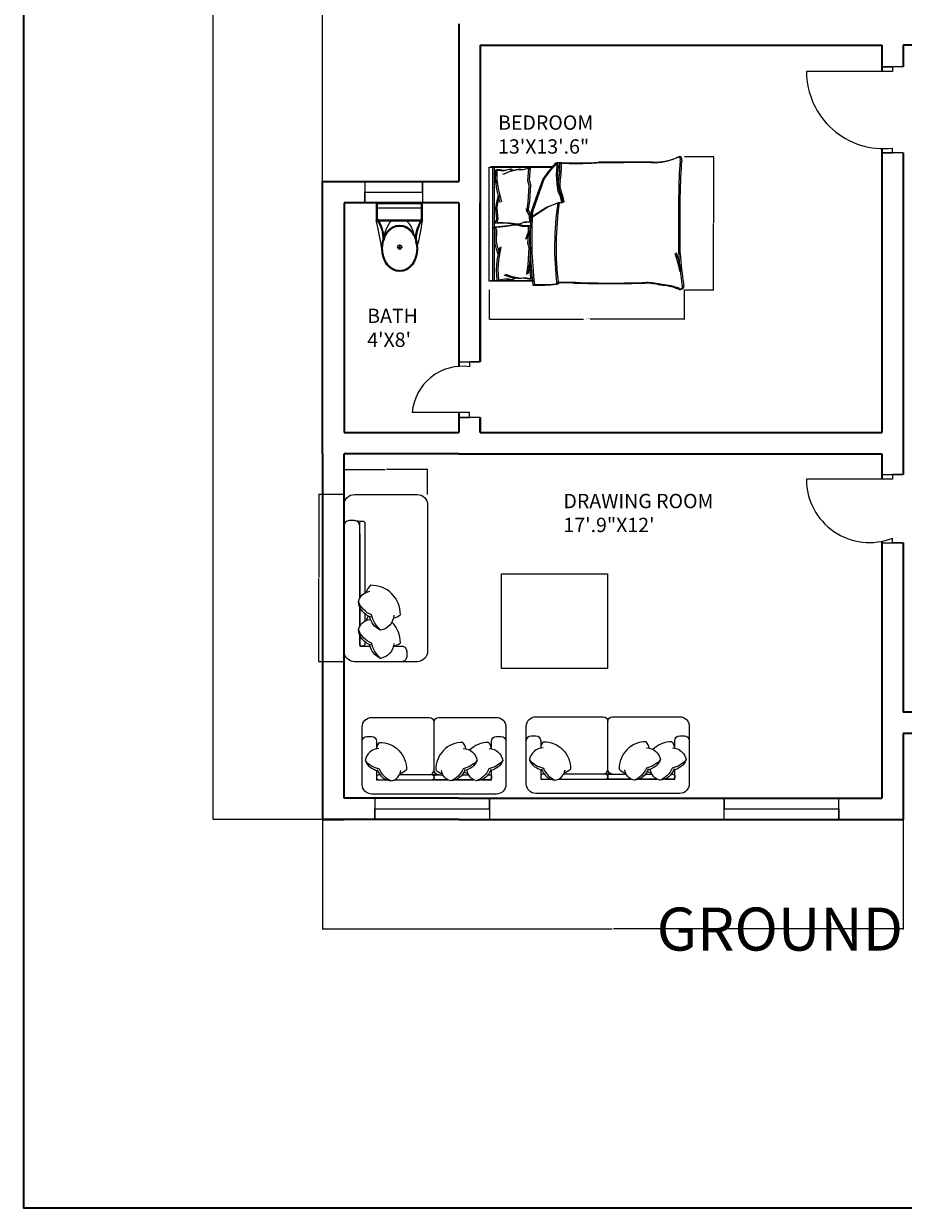
# Model space of a CAD drawing. Units: inches. Extents: x 1824 to 3509, y 619 to 2294.
# Tile 1 of 12: x 1824 to 2192, y 619 to 1115. Entities that reach past the tile are written whole.
import ezdxf

# ---------------------------------------------------------------- set-up
doc = ezdxf.new("R2010")
doc.units = ezdxf.units.IN
for name, color, linetype, lineweight in [('A-ANNO-DIMS', 2, 'Continuous', 18), ('A-ANNO-TEXT', 7, 'Continuous', 25), ('A-ANNO-TTLB', 7, 'Continuous', 35), ('A-AREA-IDEN', 7, 'Continuous', 18), ('A-DOOR', 3, 'Continuous', 18), ('A-FLOR-FIXT', 9, 'Continuous', 18), ('A-FURN', 8, 'Continuous', 13), ('A-GLAZ', 4, 'Continuous', 18), ('A-WALL', 7, 'Continuous', 35)]:
    doc.layers.add(name, color=color, linetype=linetype, lineweight=lineweight)
doc.styles.get("Standard").update_dxf_attribs({"font": 'arial.ttf'})
doc.dimstyles.get("Standard").update_dxf_attribs({"dimtxt": 0.18, "dimasz": 0.18, "dimexe": 0.18, "dimexo": 0.0625, "dimgap": 0.09, "dimtad": 0, "dimtih": 1, "dimtoh": 1, "dimdec": 4, "dimzin": 0, "dimdsep": 46, "dimtxsty": 'Standard', "dimcen": 0.09, "dimadec": 0, "dimazin": 0, "dimtfac": 1, "dimtdec": 4, "dimtofl": 0, "dimtmove": 0, "dimatfit": 3, "dimfxl": 1, "dimtolj": 1, "dimtzin": 0, "dimarcsym": 0})

# ---------------------------------------------------------------- blocks, each defined once
blk = doc.blocks.new('A$C31115884')
for p, q in [((283, 498), (223, 498)), ((258, 466), (258, 523)), ((0, 200), (0, 0)), ((520, 200), (0, 200)), ((10, 190), (10, 10)), ((510, 190), (10, 190)), ((510, 10), (510, 190)), ((520, 0), (520, 200)), ((510, 54), (0, 54)), ((10, 10), (510, 10)), ((0, 0), (520, 0))]:
    blk.add_line(p, q)
blk.add_circle((256, 496), 23.6)
for centre, radius, start, end in [((2778, -205), 2807, 165.4549, 171.7133), ((-295, 403), 365, 324.2091, 9.3499), ((-295, 403), 375, 324.2091, 9.3499), ((139, 406), 293, 315.8436, 2.6563), ((806, 403), 375, 179.2036, 215.7909), ((806, 403), 365, 170.6501, 215.7909), ((3237, 905), 2807, 188.2867, 194.5451), ((384, 406), 293, 190.2774, 224.1564)]:
    blk.add_arc(centre, radius, start, end)
blk.add_ellipse((256, 510), major_axis=(0, -261), ratio=0.772727)
blk.add_open_spline([(256, 259), (263, 259), (270, 260), (288, 262), (299, 265), (320, 273), (330, 278), (350, 291), (360, 299), (378, 316), (386, 326), (402, 347), (409, 358), (421, 383), (427, 395), (436, 422), (440, 436), (445, 465), (447, 480), (448, 509), (448, 524), (445, 553), (443, 568), (436, 596), (432, 610), (422, 636), (416, 649), (402, 672), (395, 683), (379, 703), (370, 712), (351, 728), (341, 735), (321, 746), (310, 751), (289, 757), (278, 759), (256, 761), (245, 761), (223, 757), (212, 754), (191, 746), (181, 741), (161, 728), (151, 720), (133, 703), (125, 693), (110, 672), (103, 660), (90, 636), (85, 623), (76, 596), (72, 582), (67, 553), (66, 538), (64, 509), (65, 494), (68, 465), (70, 450), (77, 422), (81, 408), (91, 382), (97, 370), (111, 346), (118, 335), (135, 316), (144, 307), (162, 291), (172, 284), (193, 273), (203, 269), (225, 262), (236, 260), (250, 259), (253, 259), (256, 259)], degree=3, knots=[0, 0, 0, 0, 0.110105, 0.110105, 0.285049, 0.285049, 0.459994, 0.459994, 0.634938, 0.634938, 0.809882, 0.809882, 0.984827, 0.984827, 1.159771, 1.159771, 1.334715, 1.334715, 1.50966, 1.50966, 1.684604, 1.684604, 1.859549, 1.859549, 2.034493, 2.034493, 2.209437, 2.209437, 2.384382, 2.384382, 2.559326, 2.559326, 2.73427, 2.73427, 2.909215, 2.909215, 3.084159, 3.084159, 3.259103, 3.259103, 3.434048, 3.434048, 3.608992, 3.608992, 3.783936, 3.783936, 3.958881, 3.958881, 4.133825, 4.133825, 4.30877, 4.30877, 4.483714, 4.483714, 4.658658, 4.658658, 4.833603, 4.833603, 5.008547, 5.008547, 5.183491, 5.183491, 5.358436, 5.358436, 5.53338, 5.53338, 5.708324, 5.708324, 5.883269, 5.883269, 6.058213, 6.058213, 6.233158, 6.233158, 6.283185, 6.283185, 6.283185, 6.283185])
blk = doc.blocks.new('DAY BED1')
at = {"color": 0}
blk.add_line((0.3, 0.25), (0.225, 0.255), dxfattribs=at)
blk.add_lwpolyline([(-0.3, 0, -0.414214), (-0.4, 0.1), (-0.4, 0.1, 0.317837), (-0.4, 0.1, -0.414214), (-0.4, 0.1), (-0.4, 0.1, 1.186185), (-0.4, 0.1, -0.414214), (-0.4, 0.1), (-0.4, 1.5, -0.414214), (-0.3, 1.6), (0.3, 1.6, -0.414214), (0.4, 1.5), (0.4, 0.1, -0.414214), (0.3, 0)], format="xyb", close=True, dxfattribs=at)
for points in [[(-0.073, 1.45), (-0.15, 1.45, -0.414214), (-0.2, 1.5), (-0.2, 1.55, -0.414214), (-0.15, 1.6)], [(-0.076, 1.425, -0.356772), (0.05, 1.568, -0.249542), (0.154, 1.438, 9.61688)], [(0.05, 1.568, -0.14773), (0.136, 1.422, -0.213343), (0.262, 1.293, -0.178662)], [(-0.073, 1.45, 0.165541), (-0.139, 1.419, 0.200231), (-0.058, 1.221, 0.121523)], [(0.143, 1.442, -0.306663), (0.262, 1.293, -0.30633), (0.154, 1.196, 0.872847)], [(0.25, 1.345), (0.25, 1.45), (0.152, 1.45, -0.414214)], [(0.2, 1.412), (0.2, 1.43, -0.414214), (0.22, 1.45), (0.23, 1.45, -0.414214), (0.25, 1.43)], [(0.25, 1.43), (0.25, 1.345, -0.414214)], [(-0.076, 1.156, -0.356772), (0.05, 1.299, -0.249542), (0.154, 1.169, 9.61688)], [(0.05, 1.299, -0.14773), (0.136, 1.153, -0.213343), (0.262, 1.024, -0.178662)], [(0.25, 1.262), (0.25, 1.075, -0.414214)], [(-0.073, 1.181, 0.165541), (-0.139, 1.15, 0.425989), (0.148, 0.869, 0.121523), (0.187, 0.936, -7.115464)], [(0.143, 1.173, -0.306663), (0.262, 1.024, -0.30633), (0.154, 0.926, 0.872847)], [(0.168, 1.163, 0.071865), (0.187, 1.205, -7.115464)], [(0.2, 1.142), (0.2, 1.211, -0.414214)], [(0.25, 0.992), (0.25, 0.275, -0.414214), (0.23, 0.255), (0.22, 0.255, -0.414214), (0.2, 0.275), (0.2, 0.942, -0.414214)], [(0.25, 0.377), (0.25, 0.3, 0.414214), (0.3, 0.25), (0.35, 0.25, 0.414214), (0.4, 0.3)]]:
    blk.add_lwpolyline(points, format="xyb", dxfattribs=at)
for points in [[(0.25, 1.075), (0.25, 1.262)], [(0.25, 0.377), (0.25, 0.992)]]:
    blk.add_lwpolyline(points, dxfattribs=at)
blk = doc.blocks.new('DOOR-BED-FRONT-36')
for p, q in [((40.5, 35.97), (31.5, 35.97)), ((31.5, 35.97), (36, 35.97)), ((36, 35.97), (36, 33.97)), ((40.5, 35.97), (40.5, 35.97)), ((36, 33.97), (0, 33.97)), ((40.5, 0), (31.5, 0)), ((31.5, 0), (31.5, 0)), ((31.5, 0), (36, 0)), ((36, 0), (36, 2))]:
    blk.add_line(p, q)
blk.add_arc((32.19, 33.97), 32.19, 180, 276.7921)
blk = doc.blocks.new('DOOR-BATH-FRONT-24')
for p, q in [((19.5, 23.21), (28.5, 23.21)), ((28.5, 23.21), (24, 23.21)), ((24, 23.21), (24, 21.21)), ((28.5, 23.21), (28.5, 23.21)), ((24, 2), (0, 2)), ((24, 0), (24, 2)), ((28.5, 0), (19.5, 0)), ((19.5, 0), (24, 0)), ((24, 0), (24, 0))]:
    blk.add_line(p, q)
blk.add_arc((21.09, 0.25), 21.16, 82.0942, 175.2586)
blk = doc.blocks.new('DOOR-DRAWING-36')
for p, q in [((36, 26.63), (0, 26.63)), ((31.55, 28.63), (37.79, 28.63)), ((40.55, 28.63), (36, 28.63)), ((36, 28.63), (36, 26.63)), ((37.79, 28.63), (40.55, 28.63)), ((36.05, 0), (36.05, 2)), ((31.55, 0), (40.55, 0)), ((40.55, 0), (36.05, 0))]:
    blk.add_line(p, q)
blk.add_arc((26.44, 26.63), 26.44, 180, 291.3224)
blk = doc.blocks.new('BED-DOUBLE-PLAN')
for p, q in [((0, 51.27), (26.61, 51.27)), ((0, 51.27), (26.61, 51.27)), ((0, 3.48), (0, 51.27)), ((0.64, 51.49), (27.25, 51.49)), ((0.64, 51.49), (27.25, 51.49)), ((1.53, 3.48), (1.53, 51.27)), ((1.53, 3.48), (1.53, 51.27)), ((2.17, 3.7), (2.17, 51.49)), ((2.17, 3.7), (2.17, 51.49)), ((2.56, 50.11), (2.46, 44.71)), ((2.56, 50.11), (2.46, 44.71)), ((2.56, 50.11), (5.77, 49.73)), ((2.56, 50.11), (5.77, 49.73)), ((3.2, 50.34), (3.1, 44.94)), ((3.2, 50.34), (3.1, 44.94)), ((3.2, 50.34), (6.41, 49.96)), ((3.2, 50.34), (6.41, 49.96)), ((5.77, 49.73), (8.34, 50.33)), ((5.77, 49.73), (8.34, 50.33)), ((6.41, 49.96), (8.98, 50.56)), ((6.41, 49.96), (8.98, 50.56)), ((11.83, 50.11), (8.26, 49.31)), ((11.83, 50.11), (8.26, 49.31)), ((8.34, 50.33), (9.38, 49.82)), ((8.34, 50.33), (9.38, 49.81)), ((12.47, 50.34), (8.9, 49.54)), ((12.47, 50.34), (8.9, 49.54)), ((8.98, 50.56), (10.02, 50.04)), ((8.98, 50.56), (10.02, 50.04)), ((13.43, 49.92), (11.83, 50.11)), ((13.43, 49.92), (11.83, 50.11)), ((14.07, 50.15), (12.47, 50.34)), ((14.07, 50.15), (12.47, 50.34)), ((16.57, 50.7), (13.43, 49.92)), ((16.57, 50.7), (13.43, 49.92)), ((17.21, 50.93), (14.07, 50.15)), ((17.21, 50.93), (14.07, 50.15)), ((16.17, 45.57), (16.57, 50.7)), ((16.17, 45.57), (16.57, 50.7)), ((16.81, 45.8), (17.21, 50.93)), ((16.81, 45.8), (17.21, 50.93)), ((27.75, 52.87), (24.5, 49.16)), ((27.75, 52.87), (24.5, 49.16)), ((28.39, 53.1), (25.13, 49.39)), ((28.39, 53.1), (25.13, 49.39)), ((29.49, 52.95), (27.75, 52.87, 3.87)), ((29.49, 52.95), (27.75, 52.87, 3.87)), ((28.36, 51.33), (27.75, 52.87)), ((28.36, 51.33), (27.75, 52.87)), ((28.06, 48.23), (28.36, 51.33)), ((28.06, 48.23), (28.36, 51.33)), ((30.13, 53.18), (28.39, 53.1, 3.87)), ((30.13, 53.18), (28.39, 53.1, 3.87)), ((29, 51.56), (28.39, 53.1)), ((29, 51.56), (28.39, 53.1)), ((28.69, 48.46), (29, 51.56)), ((28.69, 48.46), (29, 51.56)), ((2.46, 44.71), (2.54, 45.71)), ((2.46, 44.71), (2.54, 45.71)), ((2.54, 45.71), (3.07, 41.92)), ((2.54, 45.71), (3.07, 41.91)), ((3.1, 44.94), (3.18, 45.94)), ((3.1, 44.94), (3.18, 45.94)), ((3.18, 45.94), (3.71, 42.14)), ((3.18, 45.94), (3.71, 42.14)), ((8.26, 49.31), (5.58, 48.13)), ((8.26, 49.31), (5.58, 48.13)), ((8.9, 49.54), (6.22, 48.36)), ((8.9, 49.54), (6.22, 48.36)), ((16.73, 43.61), (16.17, 45.57)), ((16.73, 43.61), (16.17, 45.57)), ((17.37, 43.84), (16.81, 45.8)), ((17.37, 43.83), (16.81, 45.8)), ((22.33, 46.22), (20.32, 40.64)), ((22.33, 46.22), (20.32, 40.64)), ((22.97, 46.45), (20.96, 40.87)), ((22.97, 46.45), (20.96, 40.87)), ((24.5, 49.16), (22.33, 46.22)), ((24.5, 49.16), (22.33, 46.22)), ((25.13, 49.39), (22.97, 46.45)), ((25.13, 49.39), (22.97, 46.45)), ((28.36, 44.36), (28.06, 48.23)), ((28.36, 44.36), (28.06, 48.23)), ((29, 44.59), (28.69, 48.46)), ((29, 44.59), (28.69, 48.46)), ((3.07, 41.92), (4.42, 36.5)), ((3.07, 41.91), (4.42, 36.5)), ((3.71, 42.14), (5.06, 36.72)), ((3.71, 42.14), (5.06, 36.72)), ((16.3, 36.6), (16.73, 43.61)), ((16.3, 36.6), (16.73, 43.61)), ((16.93, 36.83), (17.37, 43.84)), ((16.93, 36.82), (17.37, 43.83)), ((20.32, 40.64), (17.38, 32.31)), ((20.32, 40.64), (17.38, 32.31)), ((20.96, 40.87), (18.02, 32.54)), ((20.96, 40.87), (18.02, 32.53)), ((28.83, 40.95), (28.36, 44.36)), ((28.83, 40.95), (28.36, 44.36)), ((29.76, 38.94), (28.83, 40.95)), ((29.76, 38.94), (28.83, 40.95)), ((29.47, 41.18), (29, 44.59)), ((29.47, 41.18), (29, 44.59)), ((30.4, 39.17), (29.47, 41.18)), ((30.4, 39.17), (29.47, 41.18)), ((79.24, 15.06), (79.24, 39.68)), ((79.24, 15.06), (79.24, 39.68)), ((79.88, 15.29), (79.88, 39.91)), ((79.88, 15.29), (79.88, 39.91)), ((3.08, 37.14), (2.54, 34.21)), ((3.08, 37.14), (2.54, 34.21)), ((3.67, 39.2), (3.08, 37.14)), ((3.67, 39.2), (3.08, 37.14)), ((3.72, 37.36), (3.18, 34.43)), ((3.72, 37.36), (3.18, 34.43)), ((4.31, 39.43), (3.72, 37.36)), ((4.31, 39.43), (3.72, 37.36)), ((15.63, 32.56), (16.3, 36.6)), ((15.63, 32.56), (16.3, 36.6)), ((16.27, 32.79), (16.93, 36.83)), ((16.27, 32.79), (16.93, 36.82)), ((23.88, 34.45), (28.36, 36.15)), ((23.88, 34.45), (28.36, 36.15)), ((24.52, 34.68), (29, 36.38)), ((24.52, 34.68), (29, 36.38)), ((28.36, 36.15), (30.38, 36.46)), ((28.36, 36.15), (30.38, 36.46)), ((29, 36.38), (31.02, 36.69)), ((29, 36.38), (31.02, 36.69)), ((30.38, 36.46), (29.76, 38.94)), ((30.38, 36.46), (29.76, 38.94)), ((31.02, 36.69), (30.4, 39.17)), ((31.02, 36.69), (30.4, 39.17)), ((2.54, 34.21), (2.56, 33.88)), ((2.54, 34.21), (2.56, 33.88)), ((2.56, 33.88), (2.98, 29.46)), ((2.56, 33.88), (2.98, 29.46)), ((3.18, 34.43), (3.2, 34.11)), ((3.18, 34.43), (3.2, 34.11)), ((3.2, 34.11), (3.62, 29.68)), ((3.2, 34.11), (3.62, 29.68)), ((16.74, 30.75), (15.45, 33.82)), ((16.74, 30.75), (15.45, 33.82)), ((17.38, 30.98), (16.09, 34.05)), ((17.38, 30.98), (16.09, 34.05)), ((16.89, 28.3), (16.74, 30.75)), ((16.89, 28.3), (16.74, 30.75)), ((17.38, 30.26), (23.88, 34.45)), ((17.38, 30.26), (23.88, 34.45)), ((17.53, 28.53), (17.38, 30.98)), ((17.53, 28.53), (17.38, 30.98)), ((18.02, 30.49), (24.52, 34.68)), ((18.02, 30.49), (24.52, 34.68)), ((1.87, 25.98), (7.22, 26.56)), ((1.87, 25.98), (7.22, 26.56)), ((2.45, 24.54), (1.87, 25.98)), ((2.45, 24.54), (1.87, 25.98)), ((2.98, 29.46), (2.49, 27.98)), ((2.98, 29.46), (2.49, 27.98)), ((2.49, 27.98), (7.87, 27.73)), ((2.49, 27.98), (7.87, 27.73)), ((2.51, 26.21), (7.86, 26.79)), ((2.51, 26.21), (7.86, 26.79)), ((3.09, 24.77), (2.51, 26.21)), ((3.09, 24.77), (2.51, 26.21)), ((3.62, 29.68), (3.13, 28.21)), ((3.62, 29.68), (3.13, 28.21)), ((3.13, 28.21), (8.51, 27.96)), ((3.13, 28.21), (8.51, 27.96)), ((7.22, 26.56), (10.4, 27.14)), ((7.22, 26.56), (10.4, 27.14)), ((7.86, 26.79), (11.04, 27.37)), ((7.86, 26.79), (11.04, 27.37)), ((7.87, 27.73), (11.08, 27.36)), ((7.87, 27.73), (11.08, 27.36)), ((8.51, 27.96), (11.72, 27.58)), ((8.51, 27.96), (11.72, 27.58)), ((10.4, 27.14), (11.7, 27.14)), ((10.4, 27.14), (11.7, 27.14)), ((11.04, 27.37), (12.34, 27.37)), ((11.04, 27.37), (12.34, 27.37)), ((11.08, 27.36), (12.38, 27.44)), ((11.08, 27.36), (12.38, 27.44)), ((11.7, 27.14), (13.58, 26.56)), ((11.7, 27.14), (13.58, 26.56)), ((11.72, 27.58), (13.02, 27.67)), ((11.72, 27.58), (13.02, 27.66)), ((12.34, 27.37), (14.22, 26.79)), ((12.34, 27.37), (14.22, 26.79)), ((12.38, 27.44), (14.22, 28.13)), ((12.38, 27.44), (14.22, 28.13)), ((13.02, 27.67), (14.86, 28.36)), ((13.02, 27.66), (14.86, 28.36)), ((13.58, 26.56), (16.26, 26.56)), ((13.58, 26.56), (16.26, 26.56)), ((14.22, 28.13), (16.89, 28.3)), ((14.22, 28.13), (16.89, 28.3)), ((14.22, 26.79), (16.9, 26.79)), ((14.22, 26.79), (16.9, 26.79)), ((14.86, 28.36), (17.53, 28.53)), ((14.86, 28.36), (17.53, 28.53)), ((16.26, 26.56), (16.26, 24.1)), ((16.26, 26.56), (16.26, 24.1)), ((16.9, 26.79), (16.9, 24.33)), ((16.9, 26.79), (16.9, 24.33)), ((2.3, 20.09), (2.45, 24.54)), ((2.3, 20.09), (2.45, 24.54)), ((2.3, 19.77), (2.3, 20.09)), ((2.3, 19.77), (2.3, 20.09)), ((2.94, 20.32), (3.09, 24.77)), ((2.94, 20.32), (3.09, 24.77)), ((2.94, 20), (2.94, 20.32)), ((2.94, 20), (2.94, 20.32)), ((3.67, 17.11), (2.94, 20)), ((3.67, 17.11), (2.94, 20)), ((16.26, 24.1), (15.17, 20.96)), ((16.26, 24.1), (15.17, 20.96)), ((16.9, 24.33), (15.81, 21.19)), ((16.9, 24.33), (15.81, 21.19)), ((16.17, 19.38), (16.57, 24.52)), ((16.17, 19.38), (16.57, 24.52)), ((16.81, 19.61), (17.21, 24.74)), ((16.81, 19.61), (17.21, 24.74)), ((3.03, 16.88), (2.3, 19.77)), ((3.03, 16.88), (2.3, 19.77)), ((3.75, 14.86), (3.03, 16.88)), ((3.75, 14.86), (3.03, 16.88)), ((3.32, 12.11), (4.33, 17.6)), ((3.32, 12.11), (4.33, 17.6)), ((4.39, 15.08), (3.67, 17.11)), ((4.39, 15.08), (3.67, 17.11)), ((3.96, 12.34), (4.97, 17.83)), ((3.96, 12.34), (4.97, 17.83)), ((16.73, 17.42), (16.17, 19.38)), ((16.73, 17.42), (16.17, 19.38)), ((16.3, 10.41), (16.73, 17.42)), ((16.3, 10.41), (16.73, 17.42)), ((17.37, 17.65), (16.81, 19.61)), ((17.37, 17.65), (16.81, 19.61)), ((16.93, 10.64), (17.37, 17.65)), ((16.93, 10.64), (17.37, 17.65)), ((3.03, 8.29), (3.32, 12.11)), ((3.03, 8.29), (3.32, 12.11)), ((3.67, 8.51), (3.96, 12.34)), ((3.67, 8.51), (3.96, 12.34)), ((15.63, 6.38), (16.3, 10.41)), ((15.63, 6.38), (16.3, 10.41)), ((16.27, 6.61), (16.93, 10.64)), ((16.27, 6.61), (16.93, 10.64)), ((16.3, 10.41), (16.62, 9.28)), ((16.3, 10.41), (16.62, 9.28)), ((16.93, 10.64), (17.26, 9.51)), ((16.93, 10.64), (17.26, 9.51)), ((3.01, 8.18), (3.03, 8.29)), ((3.01, 8.18), (3.03, 8.29)), ((3.34, 3.9), (3.01, 8.18)), ((3.34, 3.9), (3.01, 8.18)), ((3.65, 8.41), (3.67, 8.51)), ((3.65, 8.41), (3.67, 8.51)), ((3.98, 4.13), (3.65, 8.41)), ((3.98, 4.13), (3.65, 8.41)), ((8.95, 5.05), (6.21, 6.06)), ((8.95, 5.05), (6.21, 6.06)), ((9.59, 5.28), (6.85, 6.29)), ((9.59, 5.28), (6.85, 6.29)), ((12.57, 4.47), (8.95, 5.05)), ((12.57, 4.47), (8.95, 5.05)), ((13.21, 4.7), (9.59, 5.28)), ((13.21, 4.7), (9.59, 5.28)), ((14.8, 4.99), (13.21, 4.7)), ((14.8, 4.99), (13.21, 4.7)), ((17.98, 4.41), (14.8, 4.99)), ((17.98, 4.41), (14.8, 4.99)), ((16.62, 9.28), (17.34, 4.18)), ((16.62, 9.28), (17.34, 4.18)), ((17.26, 9.51), (17.98, 4.41)), ((17.26, 9.51), (17.98, 4.41)), ((18.11, 3.48), (0, 3.48)), ((18.11, 3.48), (0, 3.48)), ((18.75, 3.7), (0.64, 3.7)), ((18.75, 3.7), (0.64, 3.7)), ((3.32, 3.9), (6.5, 4.47)), ((3.32, 3.9), (6.5, 4.47)), ((3.96, 4.12), (7.14, 4.7)), ((3.96, 4.12), (7.14, 4.7)), ((6.5, 4.47), (9.1, 4.04)), ((6.5, 4.47), (9.1, 4.04)), ((7.14, 4.7), (9.74, 4.27)), ((7.14, 4.7), (9.74, 4.27)), ((9.1, 4.04), (10.11, 4.62)), ((9.1, 4.04), (10.11, 4.62)), ((9.74, 4.27), (10.75, 4.85)), ((9.74, 4.27), (10.75, 4.85)), ((14.16, 4.76), (12.57, 4.47)), ((14.16, 4.76), (12.57, 4.47)), ((17.34, 4.18), (14.16, 4.76)), ((17.34, 4.18), (14.16, 4.76))]:
    blk.add_line(p, q)
for centre, radius, start, end in [((68.67, 76.16), 23.07, 267.4714, 296.4681), ((68.67, 76.16), 23.07, 267.4714, 296.4681), ((69.31, 76.39), 23.07, 267.4714, 296.4681), ((69.31, 76.39), 23.07, 267.4714, 296.4681), ((78.87, 54.41), 1.1, 332.6588, 86.02), ((78.87, 54.41), 1.1, 332.6588, 86.02), ((79.51, 54.64), 1.1, 332.6588, 86.02), ((79.51, 54.64), 1.1, 332.6588, 86.02), ((-6.66, 51.33), 36.18, 349.8763, 2.5657), ((-6.66, 51.33), 36.18, 349.8763, 2.5657), ((36.32, 182.27), 129.5, 266.9791, 273.8365), ((36.32, 182.27), 129.5, 266.9791, 273.8365), ((-6.02, 51.56), 36.18, 349.8763, 2.5657), ((-6.02, 51.56), 36.18, 349.8763, 2.5657), ((36.95, 182.49), 129.5, 266.9791, 273.8365), ((36.95, 182.49), 129.5, 266.9791, 273.8365), ((67.82, -4508.74), 4561.86, 90.00217, 90.28689), ((67.82, -4508.74), 4561.86, 90.00217, 90.28689), ((68.46, -4508.51), 4561.86, 90.00217, 90.28689), ((68.46, -4508.51), 4561.86, 90.00217, 90.28689), ((212.28, 41.15), 133.04, 174.4998, 180.6351), ((212.28, 41.15), 133.04, 174.4998, 180.6351), ((212.92, 41.38), 133.04, 174.4998, 180.6351), ((212.92, 41.38), 133.04, 174.4998, 180.6351), ((35.07, 43.74), 6.22, 168.6608, 203.7384), ((35.07, 43.74), 6.22, 168.6608, 203.7384), ((35.71, 43.97), 6.22, 168.6608, 203.7384), ((35.71, 43.97), 6.22, 168.6608, 203.7384), ((1.48, 31.15), 29.65, 10.6617, 19.8806), ((1.48, 31.15), 29.65, 10.6617, 19.8806), ((2.12, 31.38), 29.65, 10.6617, 19.8806), ((2.12, 31.38), 29.65, 10.6617, 19.8806), ((156.32, 17.76), 129.02, 171.7845, 186.9006), ((156.32, 17.76), 129.02, 171.7845, 186.9006), ((156.96, 17.98), 129.02, 171.7845, 186.9006), ((156.96, 17.98), 129.02, 171.7845, 186.9006), ((30.44, 36.64), 0.185, 250.2464, 1.1377), ((30.44, 36.64), 0.185, 250.2464, 1.1377), ((31.08, 36.87), 0.185, 250.2464, 1.1377), ((31.08, 36.87), 0.185, 250.2464, 1.1377), ((182.05, 21.36), 164.97, 176.0865, 186.7821), ((182.05, 21.36), 164.97, 176.0865, 186.7821), ((182.69, 21.59), 164.97, 176.0865, 186.7821), ((182.69, 21.59), 164.97, 176.0865, 186.7821), ((-23.71, -17.22), 106.46, 13.3832, 17.7053), ((-23.71, -17.22), 106.46, 13.3832, 17.7053), ((-23.07, -16.99), 106.46, 13.3832, 17.7053), ((-23.07, -16.99), 106.46, 13.3832, 17.7053), ((200.84, 21.43), 121.76, 182.9958, 189.4091), ((200.84, 21.43), 121.76, 182.9958, 189.4091), ((201.48, 21.66), 121.76, 182.9958, 189.4091), ((201.48, 21.66), 121.76, 182.9958, 189.4091), ((20.1, 85.16), 83.31, 268.7218, 275.604), ((20.1, 85.16), 83.31, 268.7218, 275.604), ((20.74, 85.39), 83.31, 268.7218, 275.604), ((20.74, 85.39), 83.31, 268.7218, 275.604), ((31.17, -167.31), 170.11, 88.4762, 91.0082), ((31.17, -167.31), 170.11, 88.4762, 91.0082), ((31.81, -167.08), 170.11, 88.4762, 91.0082), ((31.81, -167.08), 170.11, 88.4762, 91.0082), ((50.61, 484.82), 482.31, 268.2277, 271.7185), ((50.61, 484.82), 482.31, 268.2277, 271.7185), ((51.25, 485.05), 482.31, 268.2277, 271.7185), ((51.25, 485.05), 482.31, 268.2277, 271.7185), ((64.52, -26.9), 29.63, 76.0648, 88.9113), ((64.52, -26.9), 29.63, 76.0648, 88.9113), ((65.15, -26.67), 29.63, 76.0648, 88.9113), ((65.15, -26.67), 29.63, 76.0648, 88.9113), ((70.28, -21.66), 23.56, 67.9751, 86.652), ((70.28, -21.66), 23.56, 67.9751, 86.652), ((70.91, -21.43), 23.56, 67.9751, 86.652), ((70.91, -21.43), 23.56, 67.9751, 86.652), ((79.72, 1.09), 1.09, 236.1736, 23.4781), ((79.72, 1.09), 1.09, 236.1736, 23.4781), ((80.36, 1.32), 1.09, 236.1736, 23.4781), ((80.36, 1.32), 1.09, 236.1736, 23.4781)]:
    blk.add_arc(centre, radius, start, end)
blk = doc.blocks.new('WIN-24')
for p, q in [((0, 0), (0, 9)), ((0, 9), (0, 4.5)), ((24, 0), (24, 9)), ((0, 4.5), (24, 4.5)), ((24, 4.5), (24, 0))]:
    blk.add_line(p, q)
blk = doc.blocks.new('WIN-48')
for p, q in [((0, 9), (0, 0)), ((48, 4.5), (48, 9)), ((48, 9), (48, 0)), ((0, 0), (0, 4.5)), ((0, 4.5), (48, 4.5))]:
    blk.add_line(p, q)
blk = doc.blocks.new('*D42')
at = {"layer": 'A-ANNO-DIMS', "color": 0, "lineweight": -2, "transparency": 16777216}
for p, q in [((2018.88, 1003.7), (2018.88, 991.35)), ((2100.43, 1003.7), (2100.43, 991.35)), ((2019.06, 991.53), (2058.29, 991.53)), ((2100.25, 991.53), (2061.02, 991.53))]:
    blk.add_line(p, q, dxfattribs=at)
at = {"layer": 'A-ANNO-DIMS', "color": 0, "transparency": 16777216}
for points in [[(2019.06, 991.56), (2019.06, 991.5), (2018.88, 991.53)], [(2100.25, 991.56), (2100.25, 991.5), (2100.43, 991.53)]]:
    blk.add_solid(points, dxfattribs=at)
at = {"layer": 'Defpoints', "color": 0, "transparency": 16777216}
for p in [(2018.88, 1003.76), (2100.43, 1003.76), (2100.43, 991.53)]:
    blk.add_point(p, dxfattribs=at)
at = {"layer": 'A-ANNO-DIMS', "color": 0, "transparency": 16777216, "insert": (2059.66, 991.53), "char_height": 0.18, "attachment_point": 5}
blk.add_mtext('\\A1;DOUBLE BED 82 TYP.', dxfattribs=at)
blk = doc.blocks.new('*D43')
at = {"layer": 'A-ANNO-DIMS', "color": 0, "lineweight": -2, "transparency": 16777216}
for p, q in [((2100.49, 1059.58), (2112.84, 1059.58)), ((2112.66, 1059.4), (2112.66, 1031.85)), ((2112.66, 1003.94), (2112.66, 1031.49)), ((2100.49, 1003.76), (2112.84, 1003.76))]:
    blk.add_line(p, q, dxfattribs=at)
at = {"layer": 'A-ANNO-DIMS', "color": 0, "transparency": 16777216}
for points in [[(2112.63, 1059.4), (2112.69, 1059.4), (2112.66, 1059.58)], [(2112.63, 1003.94), (2112.69, 1003.94), (2112.66, 1003.76)]]:
    blk.add_solid(points, dxfattribs=at)
at = {"layer": 'Defpoints', "color": 0, "transparency": 16777216}
for p in [(2100.43, 1059.58), (2112.66, 1059.58), (2100.43, 1003.76)]:
    blk.add_point(p, dxfattribs=at)
at = {"layer": 'A-ANNO-DIMS', "color": 0, "transparency": 16777216, "insert": (2112.66, 1031.67), "char_height": 0.18, "attachment_point": 5}
blk.add_mtext('\\A1;56 TYP.', dxfattribs=at)
blk = doc.blocks.new('*D92')
at = {"layer": 'A-ANNO-DIMS', "color": 0, "lineweight": -2, "transparency": 16777216}
for p, q in [((1958.03, 918.12), (1947.42, 918.12)), ((1947.6, 917.94), (1947.6, 883.33)), ((1947.6, 848.35), (1947.6, 882.96)), ((1958.03, 848.17), (1947.42, 848.17))]:
    blk.add_line(p, q, dxfattribs=at)
at = {"layer": 'A-ANNO-DIMS', "color": 0, "transparency": 16777216}
for points in [[(1947.57, 917.94), (1947.63, 917.94), (1947.6, 918.12)], [(1947.57, 848.35), (1947.63, 848.35), (1947.6, 848.17)]]:
    blk.add_solid(points, dxfattribs=at)
at = {"layer": 'Defpoints', "color": 0, "transparency": 16777216}
for p in [(1958.09, 918.12), (1947.6, 848.17), (1958.09, 848.17)]:
    blk.add_point(p, dxfattribs=at)
at = {"layer": 'A-ANNO-DIMS', "color": 0, "transparency": 16777216, "insert": (1947.6, 883.14), "char_height": 0.18, "attachment_point": 5}
blk.add_mtext('\\A1;DAY BED 70', dxfattribs=at)
blk = doc.blocks.new('*D93')
at = {"layer": 'A-ANNO-DIMS', "color": 0, "lineweight": -2, "transparency": 16777216}
for p, q in [((1958.09, 918.18), (1958.09, 928.79)), ((1958.27, 928.61), (1975.36, 928.61)), ((1992.88, 928.61), (1975.8, 928.61)), ((1993.06, 918.18), (1993.06, 928.79))]:
    blk.add_line(p, q, dxfattribs=at)
at = {"layer": 'A-ANNO-DIMS', "color": 0, "transparency": 16777216}
for points in [[(1958.27, 928.64), (1958.27, 928.58), (1958.09, 928.61)], [(1992.88, 928.64), (1992.88, 928.58), (1993.06, 928.61)]]:
    blk.add_solid(points, dxfattribs=at)
at = {"layer": 'Defpoints', "color": 0, "transparency": 16777216}
for p in [(1958.09, 928.61), (1958.09, 918.12), (1993.06, 918.12)]:
    blk.add_point(p, dxfattribs=at)
at = {"layer": 'A-ANNO-DIMS', "color": 0, "transparency": 16777216, "insert": (1975.58, 928.61), "char_height": 0.18, "attachment_point": 5}
blk.add_mtext('\\A1;35', dxfattribs=at)
blk = doc.blocks.new('*D94')
at = {"layer": 'A-ANNO-DIMS', "color": 0, "lineweight": -2, "transparency": 16777216}
for p, q in [((1949.09, 1049.16), (1949.09, 1668.03)), ((1949.27, 1667.85), (2235.8, 1667.85)), ((2522.91, 1667.85), (2236.38, 1667.85)), ((2523.09, 1622.16), (2523.09, 1668.03))]:
    blk.add_line(p, q, dxfattribs=at)
at = {"layer": 'A-ANNO-DIMS', "color": 0, "transparency": 16777216}
for points in [[(1949.27, 1667.88), (1949.27, 1667.82), (1949.09, 1667.85)], [(2522.91, 1667.88), (2522.91, 1667.82), (2523.09, 1667.85)]]:
    blk.add_solid(points, dxfattribs=at)
at = {"layer": 'Defpoints', "color": 0, "transparency": 16777216}
for p in [(2523.09, 1667.85), (2523.09, 1622.1), (1949.09, 1049.1)]:
    blk.add_point(p, dxfattribs=at)
at = {"layer": 'A-ANNO-DIMS', "color": 0, "transparency": 16777216, "insert": (2236.09, 1667.85), "char_height": 0.18, "attachment_point": 5}
blk.add_mtext('\\A1;574', dxfattribs=at)
blk = doc.blocks.new('*D95')
at = {"layer": 'A-ANNO-DIMS', "color": 0, "lineweight": -2, "transparency": 16777216}
for p, q in [((2006.03, 1622.1), (1903.16, 1622.1)), ((1903.34, 1621.92), (1903.34, 1202.28)), ((1903.34, 782.28), (1903.34, 1201.92)), ((1949.03, 782.1), (1903.16, 782.1))]:
    blk.add_line(p, q, dxfattribs=at)
at = {"layer": 'A-ANNO-DIMS', "color": 0, "transparency": 16777216}
for points in [[(1903.31, 1621.92), (1903.37, 1621.92), (1903.34, 1622.1)], [(1903.31, 782.28), (1903.37, 782.28), (1903.34, 782.1)]]:
    blk.add_solid(points, dxfattribs=at)
at = {"layer": 'Defpoints', "color": 0, "transparency": 16777216}
for p in [(1903.34, 1622.1), (2006.09, 1622.1), (1949.09, 782.1)]:
    blk.add_point(p, dxfattribs=at)
at = {"layer": 'A-ANNO-DIMS', "color": 0, "transparency": 16777216, "insert": (1903.34, 1202.1), "char_height": 0.18, "attachment_point": 5}
blk.add_mtext('\\A1;840', dxfattribs=at)
blk = doc.blocks.new('*D101')
at = {"layer": 'A-ANNO-DIMS', "color": 0, "lineweight": -2, "transparency": 16777216}
for p, q in [((1949.09, 782.04), (1949.09, 736.17)), ((2192.09, 782.04), (2192.09, 736.17)), ((1949.27, 736.35), (2070.3, 736.35)), ((2191.91, 736.35), (2070.88, 736.35))]:
    blk.add_line(p, q, dxfattribs=at)
at = {"layer": 'A-ANNO-DIMS', "color": 0, "transparency": 16777216}
for points in [[(1949.27, 736.38), (1949.27, 736.32), (1949.09, 736.35)], [(2191.91, 736.38), (2191.91, 736.32), (2192.09, 736.35)]]:
    blk.add_solid(points, dxfattribs=at)
at = {"layer": 'Defpoints', "color": 0, "transparency": 16777216}
for p in [(1949.09, 782.1), (2192.09, 782.1), (2192.09, 736.35)]:
    blk.add_point(p, dxfattribs=at)
at = {"layer": 'A-ANNO-DIMS', "color": 0, "transparency": 16777216, "insert": (2070.59, 736.35), "char_height": 0.18, "attachment_point": 5}
blk.add_mtext('\\A1;243', dxfattribs=at)

msp = doc.modelspace()

# ---------------------------------------------------------------- linework, layer by layer
at = {"layer": 'A-ANNO-TTLB'}
msp.add_lwpolyline([(1824.0608, 2293.6614), (3509.3484, 2293.6614), (3509.3484, 619.4665), (1824.0608, 619.4665)], close=True, dxfattribs=at)
at = {"layer": 'A-FURN'}
msp.add_lwpolyline([(2023.9659, 884.8904), (2068.3298, 884.8904), (2068.3298, 845.3726), (2023.9659, 845.3726)], close=True, dxfattribs=at)
at = {"layer": 'A-FURN', "ltscale": 0.03}
for points in [[(1993.7431, 824.8664, -0.41421356), (1995.7484, 822.8611, -0.41421356), (1997.7536, 824.8664), (2021.817, 824.8664, -0.41421356), (2025.8276, 820.8558), (2025.8276, 796.7924, -0.41421356), (2021.817, 792.7818), (1969.6797, 792.7818, -0.41421356), (1965.6691, 796.7924), (1965.6691, 820.8558, -0.41421356), (1969.6797, 824.8664), (1993.7431, 824.8664, -0.41421356), (1995.7484, 822.8611, -0.41421356), (1997.7536, 824.8664)], [(2066.4356, 825.1358, -0.41421356), (2068.4409, 823.1305, -0.41421356), (2070.4462, 825.1358), (2098.5201, 825.1358, -0.41421356), (2102.5307, 821.1252), (2102.5307, 797.0618, -0.41421356), (2098.5201, 793.0512), (2038.3617, 793.0512, -0.41421356), (2034.3511, 797.0618), (2034.3511, 821.1252, -0.41421356), (2038.3617, 825.1358), (2066.4356, 825.1358, -0.41421356), (2068.4409, 823.1305, -0.41421356), (2070.4462, 825.1358)]]:
    msp.add_lwpolyline(points, format="xyb", dxfattribs=at)
at = {"layer": 'A-FURN'}
for points in [[(1993.7431, 800.803, 0.41421356), (1995.7484, 802.8082), (1995.7484, 822.8611, 0.41421356)], [(1997.7536, 800.803, -0.41421356), (1995.7484, 802.8082), (1995.7484, 822.8611, -0.41421356)], [(2066.4356, 801.0724, 0.41421356), (2068.4409, 803.0776), (2068.4409, 823.1305, 0.41421356)], [(2070.4462, 801.0724, -0.41421356), (2068.4409, 803.0776), (2068.4409, 823.1305, -0.41421356)], [(1965.6691, 814.8399, -0.41421356), (1967.6744, 816.8452), (1969.6797, 816.8452, -0.41421356), (1971.685, 814.8399), (1971.685, 811.733)], [(1971.6806, 811.7321, -0.16554063), (1972.9211, 814.3817, -0.42598917), (1984.1832, 802.8941, -0.12152332), (1981.5098, 801.3107, 7.11546429)], [(2009.0137, 811.7321, 0.16554063), (2007.7732, 814.3817, 0.42598917), (1996.5112, 802.8941, 0.12152332), (1999.1846, 801.3107, -7.11546429)], [(2019.8161, 811.7321, 0.16554063), (2018.5756, 814.3817, 0.20023115), (2010.6154, 811.1548, 0.12152332)], [(2019.8118, 811.733), (2019.8118, 814.8399, -0.41421356), (2021.817, 816.8452), (2023.8223, 816.8452, -0.41421356), (2025.8276, 814.8399)], [(2034.3511, 815.1093, -0.41421356), (2036.3564, 817.1146), (2038.3617, 817.1146, -0.41421356), (2040.3669, 815.1093), (2040.3669, 812.0024)], [(2040.3626, 812.0015, -0.16554063), (2041.6031, 814.6511, -0.42598917), (2052.8652, 803.1635, -0.12152332), (2050.1918, 801.5801, 7.11546429)], [(2085.7168, 812.0015, 0.16554063), (2084.4763, 814.6511, 0.42598917), (2073.2143, 803.1635, 0.12152332), (2075.8877, 801.5801, -7.11546429)], [(2096.5192, 812.0015, 0.16554063), (2095.2787, 814.6511, 0.20023115), (2087.3185, 811.4242, 0.12152332)], [(2096.5149, 812.0024), (2096.5149, 815.1093, -0.41421356), (2098.5201, 817.1146), (2100.5254, 817.1146, -0.41421356), (2102.5307, 815.1093)], [(1972.6913, 811.8544, 0.35677236), (1966.9454, 806.7998, 0.24954205), (1972.1517, 802.6345, -9.61688035)], [(2008.003, 811.8544, -0.35677236), (2013.749, 806.7998, -0.24954205), (2008.5426, 802.6345, 9.61688035)], [(2018.8054, 811.8544, -0.35677236), (2024.5514, 806.7998, -0.24954205), (2019.345, 802.6345, 9.61688035)], [(2041.3733, 812.1238, 0.35677236), (2035.6273, 807.0692, 0.24954205), (2040.8337, 802.9039, -9.61688035)], [(2084.7061, 812.1238, -0.35677236), (2090.4521, 807.0692, -0.24954205), (2085.2457, 802.9039, 9.61688035)], [(2095.5085, 812.1238, -0.35677236), (2101.2545, 807.0692, -0.24954205), (2096.0481, 802.9039, 9.61688035)], [(1966.9454, 806.7998, 0.14772988), (1972.8062, 803.3536, 0.21334276), (1977.9776, 798.299, 0.17866181)], [(1971.9965, 803.0789, 0.30666349), (1977.9776, 798.299, 0.30632997), (1981.8848, 802.6643, -0.87284716)], [(2008.6978, 803.0789, -0.30666349), (2002.7168, 798.299, -0.30632997), (1998.8095, 802.6643, 0.87284716)], [(2013.749, 806.7998, -0.14772988), (2007.8881, 803.3536, -0.21334276), (2002.7168, 798.299, -0.17866181)], [(2019.5002, 803.0789, -0.30666349), (2013.5192, 798.299, -0.30632997), (2009.6119, 802.6643, 0.87284716)], [(2024.5514, 806.7998, -0.14772988), (2018.6905, 803.3536, -0.21334276), (2013.5192, 798.299, -0.17866181)], [(2035.6273, 807.0692, 0.14772988), (2041.4882, 803.623, 0.21334276), (2046.6595, 798.5684, 0.17866181)], [(2040.6785, 803.3483, 0.30666349), (2046.6595, 798.5684, 0.30632997), (2050.5668, 802.9337, -0.87284716)], [(2066.4356, 801.0724, 0.41421356), (2068.4409, 803.0776)], [(2070.4462, 801.0724, -0.41421356), (2068.4409, 803.0776)], [(2085.4009, 803.3483, -0.30666349), (2079.4199, 798.5684, -0.30632997), (2075.5126, 802.9337, 0.87284716)], [(2090.4521, 807.0692, -0.14772988), (2084.5912, 803.623, -0.21334276), (2079.4199, 798.5684, -0.17866181)], [(2096.2033, 803.3483, -0.30666349), (2090.2223, 798.5684, -0.30632997), (2086.315, 802.9337, 0.87284716)], [(2101.2545, 807.0692, -0.14772988), (2095.3936, 803.623, -0.21334276), (2090.2223, 798.5684, -0.17866181)], [(2092.2963, 799.0671), (2096.5149, 799.0671), (2096.5149, 803.0079, -0.41421356)], [(1973.2152, 800.803), (1972.4871, 800.803, 0.41421356), (1971.685, 800.0009), (1971.685, 799.5998, 0.41421356), (1972.4871, 798.7977)], [(1972.4871, 798.7977), (1975.9035, 798.7977, 0.41421356)], [(1979.2396, 798.7977), (1994.9463, 798.7977, 0.41421356), (1995.7484, 799.5998), (1995.7484, 800.0009, 0.41421356), (1994.9463, 800.803), (1981.2588, 800.803, 0.41421356)], [(1993.7431, 800.803, 0.41421356), (1995.7484, 802.8082)], [(1997.7536, 800.803, -0.41421356), (1995.7484, 802.8082)], [(2001.4548, 798.7977), (1996.5505, 798.7977, -0.41421356), (1995.7484, 799.5998), (1995.7484, 800.0009, -0.41421356), (1996.5505, 800.803), (1999.4356, 800.803, -0.41421356)], [(2012.2571, 798.7977), (2004.7908, 798.7977, -0.41421356)], [(2007.4791, 800.803), (2010.2379, 800.803, -0.41421356)], [(2008.3057, 802.0947, 0.07186538), (2009.9869, 801.3107, -7.11546429)], [(2015.5932, 798.7977), (2019.8118, 798.7977), (2019.8118, 802.7385, -0.41421356)], [(2019.0096, 798.7977), (2015.5932, 798.7977, -0.41421356)], [(2018.2815, 800.803), (2019.0096, 800.803, -0.41421356), (2019.8118, 800.0009), (2019.8118, 799.5998, -0.41421356), (2019.0096, 798.7977)], [(2041.8972, 801.0724), (2041.1691, 801.0724, 0.41421356), (2040.3669, 800.2703), (2040.3669, 799.8692, 0.41421356), (2041.1691, 799.0671)], [(2041.1691, 799.0671), (2044.5855, 799.0671, 0.41421356)], [(2047.9216, 799.0671), (2067.6388, 799.0671, 0.41421356), (2068.4409, 799.8692), (2068.4409, 800.2703, 0.41421356), (2067.6388, 801.0724), (2049.9408, 801.0724, 0.41421356)], [(2078.1579, 799.0671), (2069.243, 799.0671, -0.41421356), (2068.4409, 799.8692), (2068.4409, 800.2703, -0.41421356), (2069.243, 801.0724), (2076.1387, 801.0724, -0.41421356)], [(2088.9602, 799.0671), (2081.4939, 799.0671, -0.41421356)], [(2084.1822, 801.0724), (2086.941, 801.0724, -0.41421356)], [(2085.0088, 802.3641, 0.07186538), (2086.69, 801.5801, -7.11546429)], [(2095.7127, 799.0671), (2092.2963, 799.0671, -0.41421356)], [(2094.9846, 801.0724), (2095.7127, 801.0724, -0.41421356), (2096.5149, 800.2703), (2096.5149, 799.8692, -0.41421356), (2095.7127, 799.0671)]]:
    msp.add_lwpolyline(points, format="xyb", dxfattribs=at)
for points in [[(2040.3669, 803.0079), (2040.3669, 799.0671), (2044.5855, 799.0671)], [(1971.685, 802.7385), (1971.685, 798.7977), (1975.9035, 798.7977)], [(1979.2396, 798.7977), (2001.4548, 798.7977)], [(2004.7908, 798.7977), (2012.2571, 798.7977)], [(2047.9216, 799.0671), (2078.1579, 799.0671)], [(2081.4939, 799.0671), (2088.9602, 799.0671)]]:
    msp.add_lwpolyline(points, dxfattribs=at)
for points in [[(1994.9463, 798.7977), (1996.5505, 798.7977, -0.41421356), (1995.7484, 799.5998), (1995.7484, 800.0009, -0.41421356), (1996.5505, 800.803), (1994.9463, 800.803, -0.41421356), (1995.7484, 800.0009), (1995.7484, 799.5998, -0.41421356)], [(2067.6388, 799.0671), (2069.243, 799.0671, -0.41421356), (2068.4409, 799.8692), (2068.4409, 800.2703, -0.41421356), (2069.243, 801.0724), (2067.6388, 801.0724, -0.41421356), (2068.4409, 800.2703), (2068.4409, 799.8692, -0.41421356)]]:
    msp.add_lwpolyline(points, format="xyb", close=True, dxfattribs=at)
at = {"layer": 'A-GLAZ'}
msp.add_line((2117.1111, 791.1012), (2117.1111, 791.1012), dxfattribs=at)
at = {"layer": 'A-WALL'}
for p, q in [((2006.0899, 1115.1012), (2006.0899, 1049.1012)), ((2015.0899, 1106.1012), (2183.0899, 1106.1012)), ((2015.0899, 1106.1012), (2015.0899, 973.58)), ((2183.0899, 1106.1012), (2183.0899, 1095.0468)), ((2192.0899, 1106.1012), (2192.0899, 1097.0468)), ((2222.4401, 1106.1012), (2192.0899, 1106.1012)), ((2183.0899, 1062.8616), (2183.0899, 944.1012)), ((2192.0899, 1061.08), (2192.0899, 926.4727)), ((1949.0899, 1040.1012), (1949.0899, 1049.1012)), ((1949.0899, 1049.1012), (2006.0899, 1049.1012)), ((1949.0899, 935.1012), (1949.0899, 1040.1012)), ((1967.0899, 1040.1012), (1958.0899, 1040.1012)), ((1958.0899, 1040.1012), (1958.0899, 944.1012)), ((2006.0899, 1040.1012), (1967.0899, 1040.1012)), ((2006.0899, 1040.1012), (2006.0899, 971.7214)), ((2015.0899, 973.58), (2015.0899, 1040.1012)), ((2006.0899, 952.3686), (2006.0899, 944.1012)), ((2015.0899, 944.1012), (2015.0899, 950.3686)), ((2015.0899, 950.3686), (2015.0899, 944.1012)), ((1958.0899, 944.1012), (2006.0899, 944.1012)), ((2015.0899, 944.1012), (2183.0899, 944.1012)), ((1949.0899, 935.1012), (1949.0899, 782.1012)), ((2006.0899, 935.1012), (1958.0899, 935.1012)), ((1958.0899, 791.1012), (1958.0899, 935.1012)), ((2006.0899, 935.1012), (2183.0899, 935.1012)), ((2006.0899, 935.1012), (2006.0899, 935.1012)), ((2183.0899, 935.1012), (2183.0899, 924.4727)), ((2183.0899, 898.5364), (2183.0899, 791.1012)), ((2192.0899, 897.8469), (2192.0899, 827.1012)), ((2203.9846, 827.1012), (2192.0899, 827.1012)), ((2192.0899, 818.1012), (2192.0899, 782.1012)), ((2201.9846, 818.1012), (2192.0899, 818.1012)), ((2006.0899, 791.1012), (1958.0899, 791.1012)), ((2006.0899, 791.1012), (2183.0899, 791.1012)), ((1958.0899, 782.1012), (1949.0899, 782.1012)), ((1949.0899, 782.1012), (1958.0899, 782.1012)), ((2006.0899, 782.1012), (1958.0899, 782.1012)), ((2006.0899, 782.1012), (2192.0899, 782.1012))]:
    msp.add_line(p, q, dxfattribs=at)

# ---------------------------------------------------------------- block references
at = {"layer": 'A-DOOR'}
for name, p in [('DOOR-BED-FRONT-36', (2151.59, 1061.08)), ('DOOR-BATH-FRONT-24', (1986.59, 950.369)), ('DOOR-DRAWING-36', (2151.542, 897.847))]:
    msp.add_blockref(name, p, dxfattribs=at)
at = {"layer": 'A-FLOR-FIXT', "xscale": 0.0372717239612423, "yscale": 0.0372717239612423, "zscale": 0.0372717239612423, "rotation": 180}
msp.add_blockref('A$C31115884', (1990.9204, 1040.1012), dxfattribs=at)
at = {"layer": 'A-FURN'}
msp.add_blockref('BED-DOUBLE-PLAN', (2018.8816, 1003.8439), dxfattribs=at)
at = {"layer": 'A-FURN', "ltscale": 0.03, "xscale": 43.71736627048695, "yscale": 43.71736627048695, "zscale": 43.71736627048695, "rotation": 180.0000000006138}
msp.add_blockref('DAY BED1', (1975.5769, 918.1178), dxfattribs=at)
at = {"layer": 'A-GLAZ', "extrusion": (0, 0, -1), "zscale": -1, "rotation": 180}
for name, p in [('WIN-24', (-1966.8614, 1049.1013)), ('WIN-48', (-2117.1113, 791.1013))]:
    msp.add_blockref(name, p, dxfattribs=at)
at = {"layer": 'A-GLAZ'}
msp.add_blockref('WIN-48', (1970.9534, 782.101), dxfattribs=at)

# ---------------------------------------------------------------- texts
at = {"layer": 'A-ANNO-TEXT', "insert": (2088.9129, 745.2888), "char_height": 18, "attachment_point": 1}
msp.add_mtext_dynamic_manual_height_columns('GROUND FLOOR PLAN', width=638.440451, gutter_width=12.5, heights=[0], dxfattribs=at)
at = {"layer": 'A-AREA-IDEN', "char_height": 6, "attachment_point": 1}
for s, width, insert in [('BEDROOM\\P13\'X13\'.6"', 153.560286, (2022.546, 1076.7356)), ('DRAWING ROOM\\P17\'.9"X12\'', 144.902175, (2049.8893, 918.3839))]:
    msp.add_mtext_dynamic_manual_height_columns(s, width=width, gutter_width=12.5, heights=[0], dxfattribs=dict(at, insert=insert))
at = {"layer": 'A-AREA-IDEN', "insert": (1967.7893, 995.8681), "char_height": 6, "width": 43.729864, "attachment_point": 1}
msp.add_mtext("BATH\\P4'X8'", dxfattribs=at)

# ---------------------------------------------------------------- dimensions: what is measured, and where the dimension line sits
at = {"layer": 'A-ANNO-DIMS'}
for base, p1, p2, picture, middle in [((2523.0899, 1667.8512), (1949.0899, 1049.1012), (2523.0899, 1622.1012), '*D94', (2236.0899, 1667.8512)), ((2192.0899, 736.3512), (1949.0899, 782.1012), (2192.0899, 782.1012), '*D101', (2070.5899, 736.3512))]:
    dim = msp.add_linear_dim(base=base, p1=p1, p2=p2, dimstyle='Standard', override={"dimdec": 0, "dimlfac": 1, "dimrnd": 0, "dimzin": 0, "dimdsep": 46, "dimlunit": 2}, dxfattribs=at)
    dim.commit()
    dim.dimension.update_dxf_attribs({"geometry": picture, "text_midpoint": middle})
for base, p1, p2, angle, picture, middle in [((1903.3399, 1622.1012), (1949.0899, 782.1012), (2006.0899, 1622.1012), 90, '*D95', (1903.3399, 1202.1012)), ((1958.0899, 928.61), (1993.0638, 918.1178), (1958.0899, 918.1178), 180, '*D93', (1975.5769, 928.61))]:
    dim = msp.add_linear_dim(base=base, p1=p1, p2=p2, angle=angle, dimstyle='Standard', override={"dimdec": 0, "dimlfac": 1, "dimrnd": 0, "dimzin": 0, "dimdsep": 46, "dimlunit": 2}, dxfattribs=at)
    dim.commit()
    dim.dimension.update_dxf_attribs({"geometry": picture, "text_midpoint": middle})
for base, p1, p2, angle, text, picture, middle in [((2112.6624, 1059.5826), (2100.4301, 1003.7581), (2100.4301, 1059.5826), 90, '<> TYP.', '*D43', (2112.6624, 1031.6703)), ((1947.5977, 848.1701), (1958.0899, 918.1178), (1958.0899, 848.1701), 270, 'DAY BED <>', '*D92', (1947.5977, 883.1439))]:
    dim = msp.add_linear_dim(base=base, p1=p1, p2=p2, angle=angle, text=text, dimstyle='Standard', override={"dimdec": 0, "dimlfac": 1, "dimrnd": 0, "dimzin": 0, "dimdsep": 46, "dimlunit": 2}, dxfattribs=at)
    dim.commit()
    dim.dimension.update_dxf_attribs({"geometry": picture, "text_midpoint": middle})
dim = msp.add_linear_dim(base=(2100.4301, 991.5258), p1=(2018.8814, 1003.7581), p2=(2100.4301, 1003.7581), text='DOUBLE BED <> TYP.', dimstyle='Standard', override={"dimdec": 0, "dimlfac": 1, "dimrnd": 0, "dimzin": 0, "dimdsep": 46, "dimlunit": 2}, dxfattribs=at)
dim.commit()
dim.dimension.update_dxf_attribs({"geometry": '*D42', "text_midpoint": (2059.6557, 991.5258)})

doc.saveas('drawing.dxf')
